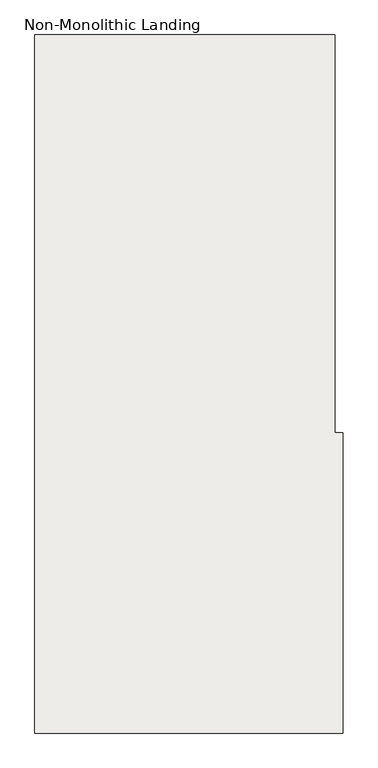
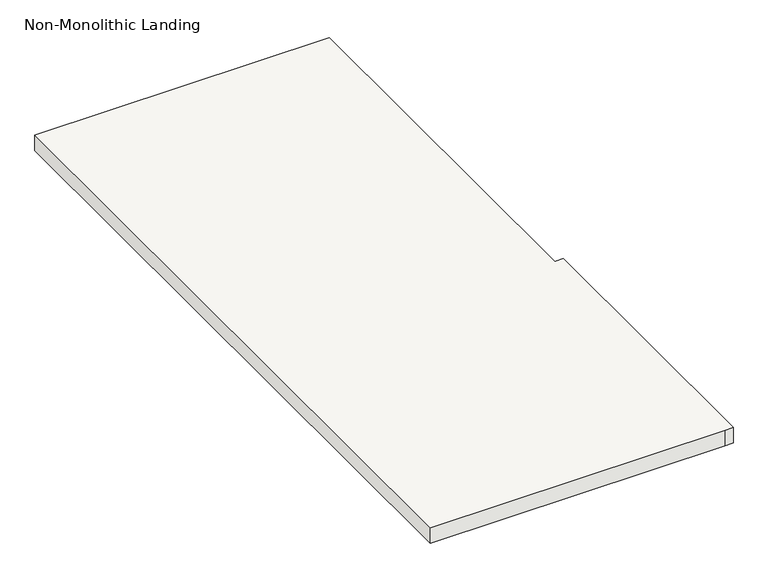
"""IFC4 building model written with IfcOpenShell, lengths in millimetres: slab geometry, Non-Monolithic Landing."""

from ifc_helpers import new_model, si_unit, origin, place, context, project, spatial, faceted_brep, source, transform, mapped, element, save


def non_monolithic_landing_255cec53(model_context):
    return source(origin(), model_context, "Body", "Brep", [
        faceted_brep([(-8810.2517085, 2919.0826226, 8523.8166667), (-8784.8517085, 2919.0826226, 8549.2166667), (-8784.8517085, 2004.6826226, 8549.2166667), (-8810.2517085, 2004.6826226, 8523.8166667), (-9699.2517085, 2919.0826226, 8568.2666667), (-9699.2517085, 792.0165128, 8568.2666667), (-8784.8517085, 792.0165128, 8568.2666667), (-8759.4517085, 792.0165128, 8568.2666667), (-8759.4517085, 1706.4165128, 8568.2666667), (-8784.8517085, 1706.4165128, 8568.2666667), (-8784.8517085, 2919.0826226, 8568.2666667), (-8810.2517085, 2004.6826226, 8517.4666667), (-8784.8517085, 2004.6826226, 8517.4666667), (-8784.8517085, 1706.4165128, 8517.4666667), (-8759.4517085, 1706.4165128, 8517.4666667), (-8759.4517085, 792.0165128, 8517.4666667), (-8784.8517085, 792.0165128, 8517.4666667), (-9699.2517085, 792.0165128, 8517.4666667), (-9699.2517085, 2919.0826226, 8517.4666667), (-8810.2517085, 2919.0826226, 8517.4666667)], [[[0, 1, 2, 3]], [[4, 5, 6, 7, 8, 9, 10]], [[11, 12, 13, 14, 15, 16, 17, 18, 19]], [[12, 11, 3, 2]], [[11, 19, 0, 3]], [[4, 10, 1, 0, 19, 18]], [[5, 4, 18, 17]], [[6, 5, 17, 16]], [[7, 6, 16, 15]], [[8, 7, 15, 14]], [[9, 8, 14, 13]], [[10, 9, 13, 12, 2, 1]]]),
    ])


if __name__ == "__main__":
    model = new_model("IFC4")
    model_context = context("Model", 3, world=origin())
    ifc_project = project(units=[si_unit("LENGTHUNIT", "METRE", prefix="MILLI")], contexts=[model_context])
    site = spatial("IfcSite", under=ifc_project)
    building = spatial("IfcBuilding", under=site)
    placement = place(None, origin())
    non_monolithic_landing_shape = non_monolithic_landing_255cec53(model_context)
    element("IfcSlab", 1, ObjectType="Non-Monolithic Landing", at=placement, inside=building, context=model_context, shape_type="MappedRepresentation", body=[
        mapped(non_monolithic_landing_shape, transform((0.0, 0.0, 0.0), x_axis=(1.0, 0.0, 0.0), y_axis=(0.0, 1.0, 0.0), z_axis=(0.0, 0.0, 1.0))),
    ])
    save(model, "model.ifc")
